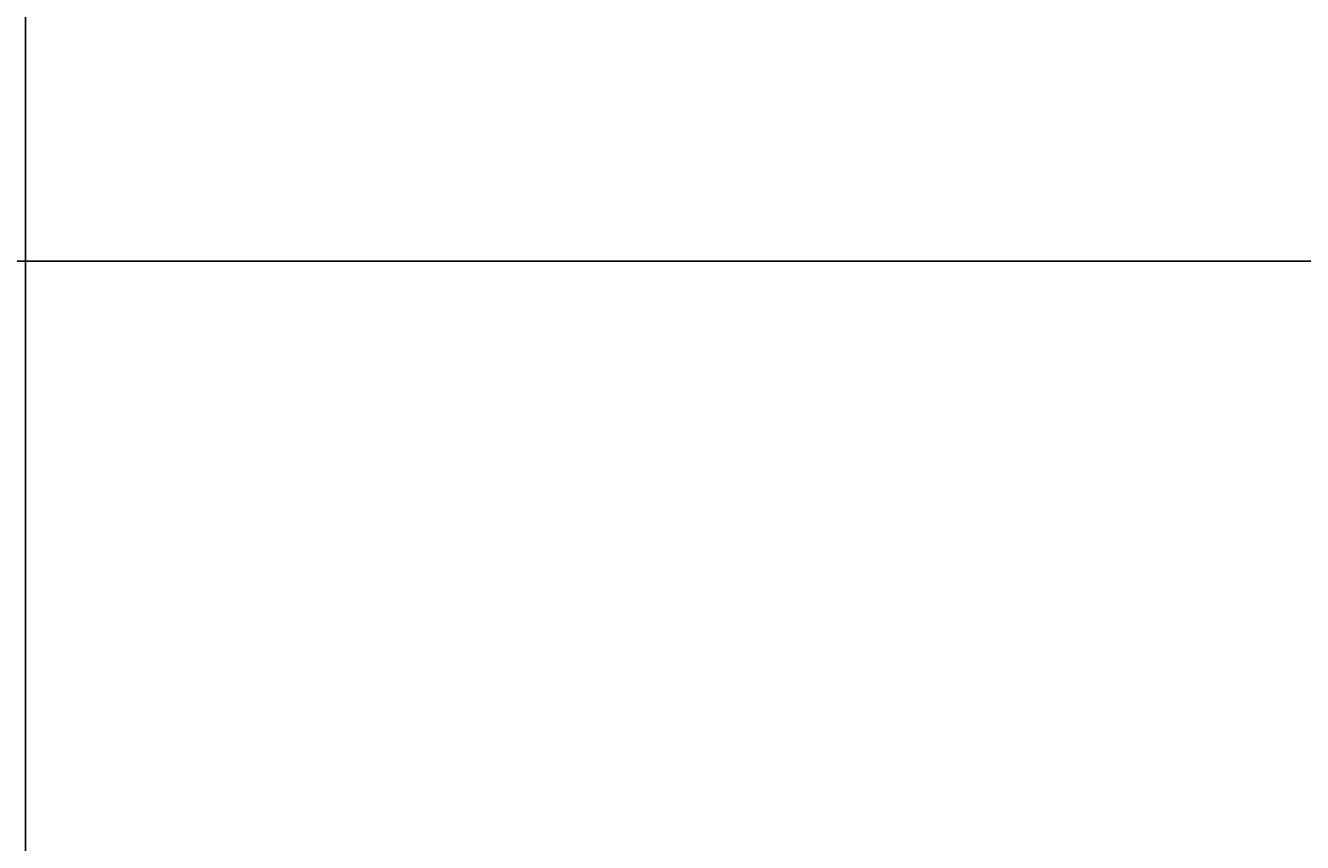
# Model space of a CAD drawing. Units: inches. Extents: x 35362 to 73946, y 43607 to 67532.
# Tile 134 of 134: x 67327 to 68296, y 56407 to 57027. Entities that reach past the tile are written whole.
import ezdxf

# ---------------------------------------------------------------- set-up
doc = ezdxf.new("R2010")
doc.units = ezdxf.units.IN
doc.header["$MEASUREMENT"] = 0
doc.layers.add('A-ANNO-DIMS', color=2, linetype='Continuous', lineweight=18)
doc.styles.get("Standard").update_dxf_attribs({"font": 'arial.ttf'})
doc.dimstyles.get("Standard").update_dxf_attribs({"dimtxt": 0.18, "dimasz": 0.18, "dimexe": 0.18, "dimexo": 0.0625, "dimgap": 0.09, "dimtad": 0, "dimtih": 1, "dimtoh": 1, "dimdec": 4, "dimzin": 0, "dimdsep": 46, "dimtxsty": 'Standard', "dimcen": 0.09, "dimadec": 0, "dimazin": 0, "dimtfac": 1, "dimtdec": 4, "dimtofl": 0, "dimtmove": 0, "dimatfit": 3, "dimfxl": 1, "dimtolj": 1, "dimtzin": 0, "dimarcsym": 0})

# ---------------------------------------------------------------- blocks, each defined once
blk = doc.blocks.new('*D8')
at = {"layer": 'A-ANNO-DIMS', "color": 0, "lineweight": -2, "transparency": 16777216}
for p, q in [((66271.28651900003, 65771.51172800003), (73945.82566600003, 65771.51172800003)), ((73945.64566600005, 65771.33172800003), (73945.64566600005, 59737.03093663782)), ((73945.64566600005, 53702.36633900002), (73945.64566600005, 59736.66713036224)), ((72185.70816600003, 53702.18633900003), (73945.82566600003, 53702.18633900003))]:
    blk.add_line(p, q, dxfattribs=at)
at = {"layer": 'A-ANNO-DIMS', "color": 0, "transparency": 16777216}
for points in [[(73945.61566600006, 65771.33172800003), (73945.67566600005, 65771.33172800003), (73945.64566600005, 65771.51172800003)], [(73945.61566600006, 53702.36633900002), (73945.67566600005, 53702.36633900002), (73945.64566600005, 53702.18633900003)]]:
    blk.add_solid(points, dxfattribs=at)
at = {"layer": 'Defpoints', "color": 0, "transparency": 16777216}
for p in [(66271.22401900003, 65771.51172800003), (73945.64566600005, 65771.51172800003), (72185.64566600003, 53702.18633900003)]:
    blk.add_point(p, dxfattribs=at)
at = {"layer": 'A-ANNO-DIMS', "color": 0, "transparency": 16777216, "insert": (73945.64566600005, 59736.84903349999), "char_height": 0.18, "attachment_point": 5}
blk.add_mtext('\\A1;12069', dxfattribs=at)
blk = doc.blocks.new('*D10')
at = {"layer": 'A-ANNO-DIMS', "color": 0, "lineweight": -2, "transparency": 16777216}
for p, q in [((61240.96983600002, 59185.14395700003), (73945.82566600003, 59185.14395700003)), ((73945.64566600005, 59184.96395700003), (73945.64566600005, 56268.51827402935)), ((73945.64566600005, 53351.70866200003), (73945.64566600005, 56268.1543449707)), ((61240.96983600002, 53351.52866200003), (73945.82566600003, 53351.52866200003))]:
    blk.add_line(p, q, dxfattribs=at)
at = {"layer": 'A-ANNO-DIMS', "color": 0, "transparency": 16777216}
for points in [[(73945.61566600006, 59184.96395700003), (73945.67566600005, 59184.96395700003), (73945.64566600005, 59185.14395700003)], [(73945.61566600006, 53351.70866200003), (73945.67566600005, 53351.70866200003), (73945.64566600005, 53351.52866200003)]]:
    blk.add_solid(points, dxfattribs=at)
at = {"layer": 'Defpoints', "color": 0, "transparency": 16777216}
for p in [(61240.90733600002, 59185.14395700003), (61240.90733600002, 53351.52866200003), (73945.64566600005, 53351.52866200003)]:
    blk.add_point(p, dxfattribs=at)
at = {"layer": 'A-ANNO-DIMS', "color": 0, "transparency": 16777216, "insert": (73945.64566600005, 56268.33630949999), "char_height": 0.18, "attachment_point": 5}
blk.add_mtext('\\A1;5834', dxfattribs=at)
blk = doc.blocks.new('*D36')
at = {"layer": 'A-ANNO-DIMS', "color": 0, "lineweight": -2, "transparency": 16777216}
for p, q in [((68320.80826200004, 60122.34633200002), (35361.76908500003, 60122.34633200002)), ((35361.94908500003, 60122.16633200002), (35361.94908500003, 57247.82893113781)), ((35361.94908500003, 54373.12772400002), (35361.94908500003, 57247.46512486223)), ((68320.80826200004, 54372.94772400003), (35361.76908500003, 54372.94772400002))]:
    blk.add_line(p, q, dxfattribs=at)
at = {"layer": 'A-ANNO-DIMS', "color": 0, "transparency": 16777216}
for points in [[(35361.91908500003, 60122.16633200002), (35361.97908500003, 60122.16633200002), (35361.94908500003, 60122.34633200002)], [(35361.91908500003, 54373.12772400002), (35361.97908500003, 54373.12772400002), (35361.94908500003, 54372.94772400002)]]:
    blk.add_solid(points, dxfattribs=at)
at = {"layer": 'Defpoints', "color": 0, "transparency": 16777216}
for p in [(68320.87076200004, 60122.34633200002), (35361.94908500003, 54372.94772400002), (68320.87076200004, 54372.94772400003)]:
    blk.add_point(p, dxfattribs=at)
at = {"layer": 'A-ANNO-DIMS', "color": 0, "transparency": 16777216, "insert": (35361.94908500004, 57247.64702799999), "char_height": 0.18, "attachment_point": 5}
blk.add_mtext('\\A1;5749.4', dxfattribs=at)
blk = doc.blocks.new('*D47')
at = {"layer": 'A-ANNO-DIMS', "color": 0, "lineweight": -2, "transparency": 16777216}
for p, q in [((50339.58680000003, 58279.98849500002), (73945.82566600003, 58279.98849500002)), ((73945.64566600005, 58279.80849500002), (73945.64566600005, 57564.17141502935)), ((73945.64566600005, 56848.17040600003), (73945.64566600005, 57563.80748597069)), ((50339.58680000003, 56847.99040600003), (73945.82566600003, 56847.99040600003))]:
    blk.add_line(p, q, dxfattribs=at)
at = {"layer": 'A-ANNO-DIMS', "color": 0, "transparency": 16777216}
for points in [[(73945.61566600006, 58279.80849500002), (73945.67566600005, 58279.80849500002), (73945.64566600005, 58279.98849500002)], [(73945.61566600006, 56848.17040600003), (73945.67566600005, 56848.17040600003), (73945.64566600005, 56847.99040600003)]]:
    blk.add_solid(points, dxfattribs=at)
at = {"layer": 'Defpoints', "color": 0, "transparency": 16777216}
for p in [(50339.52430000002, 58279.98849500002), (50339.52430000002, 56847.99040600003), (73945.64566600005, 56847.99040600003)]:
    blk.add_point(p, dxfattribs=at)
at = {"layer": 'A-ANNO-DIMS', "color": 0, "transparency": 16777216, "insert": (73945.64566600005, 57563.98945049999), "char_height": 0.18, "attachment_point": 5}
blk.add_mtext('\\A1;1432.0', dxfattribs=at)
blk = doc.blocks.new('*D65')
at = {"layer": 'A-ANNO-DIMS', "color": 0, "lineweight": -2, "transparency": 16777216}
for p, q in [((65336.01600799999, 61293.223552), (65336.01600799999, 43606.678996)), ((67326.639741, 61293.223552), (67326.639741, 43606.678996)), ((65336.19600799999, 43606.858996), (66330.87277900206, 43606.858996)), ((67326.45974100001, 43606.858996), (66331.78296999796, 43606.858996))]:
    blk.add_line(p, q, dxfattribs=at)
at = {"layer": 'A-ANNO-DIMS', "color": 0, "transparency": 16777216}
for points in [[(65336.19600799999, 43606.888996), (65336.19600799999, 43606.828996), (65336.01600799999, 43606.858996)], [(67326.45974100001, 43606.888996), (67326.45974100001, 43606.828996), (67326.639741, 43606.858996)]]:
    blk.add_solid(points, dxfattribs=at)
at = {"layer": 'Defpoints', "color": 0, "transparency": 16777216}
for p in [(65336.01600799999, 61293.286052), (67326.639741, 61293.286052), (67326.639741, 43606.858996)]:
    blk.add_point(p, dxfattribs=at)
at = {"layer": 'A-ANNO-DIMS', "color": 0, "transparency": 16777216, "insert": (66331.32787450001, 43606.858996), "char_height": 0.18, "attachment_point": 5}
blk.add_mtext('\\A1;1990.6', dxfattribs=at)

msp = doc.modelspace()

# ---------------------------------------------------------------- dimensions: what is measured, and where the dimension line sits
at = {"layer": 'A-ANNO-DIMS'}
for base, p1, p2, override, picture, middle in [((73945.64566600005, 65771.51172800003), (72185.645666, 53702.186339), (66271.224019, 65771.51172799998), {"dimdec": 0, "dimlfac": 1, "dimrnd": 0, "dimzin": 0, "dimdsep": 46, "dimlunit": 2}, '*D8', (73945.64566600005, 59736.84903349999)), ((35361.94908500003, 54372.94772400002), (68320.870762, 60122.346332), (68320.870762, 54372.947724), {"dimdec": 1, "dimlfac": 1, "dimrnd": 0, "dimzin": 0, "dimdsep": 46, "dimlunit": 2}, '*D36', (35361.94908500004, 57247.64702799999)), ((73945.64566600005, 53351.52866200003), (61240.907336, 59185.14395699999), (61240.907336, 53351.52866199999), {"dimdec": 0, "dimlfac": 1, "dimrnd": 0, "dimzin": 0, "dimdsep": 46, "dimlunit": 2}, '*D10', (73945.64566600005, 56268.33630949999)), ((73945.64566600005, 56847.99040600003), (50339.5243, 58279.988495), (50339.5243, 56847.99040599999), {"dimdec": 1, "dimlfac": 1, "dimrnd": 0, "dimzin": 0, "dimdsep": 46, "dimlunit": 2}, '*D47', (73945.64566600005, 57563.98945049999))]:
    dim = msp.add_linear_dim(base=base, p1=p1, p2=p2, angle=90, dimstyle='Standard', override=override, dxfattribs=at)
    dim.commit()
    dim.dimension.update_dxf_attribs({"geometry": picture, "text_midpoint": middle})
dim = msp.add_linear_dim(base=(67326.639741, 43606.858996), p1=(65336.01600799999, 61293.286052), p2=(67326.639741, 61293.286052), dimstyle='Standard', override={"dimdec": 1, "dimlfac": 1, "dimrnd": 0, "dimzin": 0, "dimdsep": 46, "dimlunit": 2}, dxfattribs=at)
dim.commit()
dim.dimension.update_dxf_attribs({"geometry": '*D65', "text_midpoint": (66331.32787450001, 43606.858996)})

doc.saveas('drawing.dxf')
